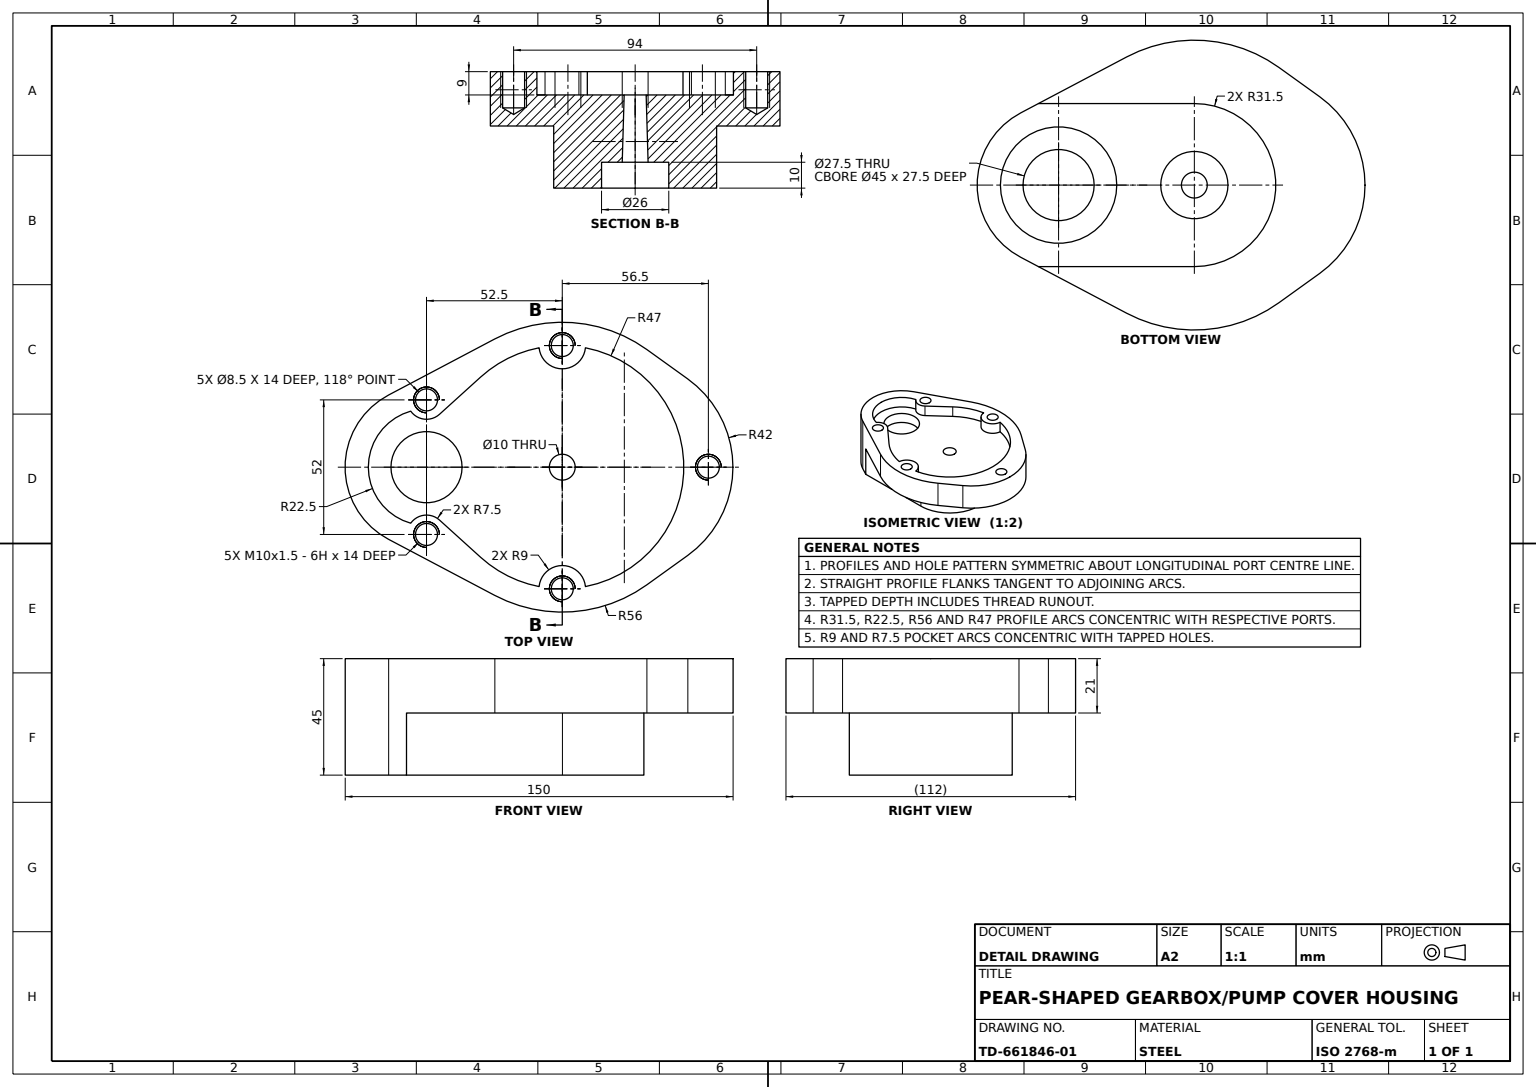
from build123d import *

# Parameters (mm, degrees)
FLANGE_BASE_21MM_DEPTH               = 21
PORT_POCKET_9MM_DEEP_DEPTH           = 9
TAPPED_HOLE_M10_DRILL_8_5_D          = 8.5
TAPPED_HOLE_M10_DRILL_8_5_DEPTH      = 14
TAPPED_HOLE_M10_DRILL_8_5_TIP        = 2.553657631
PORT_START                           = 24
PORT_BOSS_24MM_DEPTH                 = 24
SECONDARY_PORT_C_BORE_10_D           = 10
SECONDARY_PORT_C_BORE_10_DEPTH       = 99.679486355
SECONDARY_PORT_C_BORE_10_CBORE_D     = 26
SECONDARY_PORT_C_BORE_10_CBORE_DEPTH = 10


with BuildPart() as part:
    # Flange Base Profile → Flange Base 21mm (new body)
    with BuildSketch(Plane(origin=(0, 0, 0), x_dir=(1, 0, 0), z_dir=(0, 1, 0))):
        with BuildLine():
            Line((-49.528263536, 26.366666667), (-27.859648239, -14.7))
            ThreePointArc((-27.859648239, -14.7), (0, -31.5), (27.859648239, -14.7))
            Line((27.859648239, -14.7), (49.528263536, 26.366666667))
            ThreePointArc((49.528263536, 26.366666667), (55.868076531, 56.341617458), (45.485040276, 85.166666667))
            Line((45.485040276, 85.166666667), (34.113780207, 101))
            ThreePointArc((34.113780207, 101), (0, 118.5), (-34.113780207, 101))
            Line((-34.113780207, 101), (-45.485040276, 85.166666667))
            ThreePointArc((-45.485040276, 85.166666667), (-55.868076531, 56.341617458), (-49.528263536, 26.366666667))
        make_face()
    extrude(amount=FLANGE_BASE_21MM_DEPTH)

    # Port Pocket Profile → Port Pocket 9mm Deep (cut)
    with BuildSketch(Plane(origin=(0, 21, 0), x_dir=(1, 0, 0), z_dir=(0, 1, 0))):
        with BuildLine():
            Line((-21.596473004, 6.312079988), (-20.437807431, 5.031104632))
            ThreePointArc((-20.437807431, 5.031104632), (-18.544261668, -0.813612883), (-21.653846154, -6.112360162))
            ThreePointArc((-21.653846154, -6.112360162), (0, -22.5), (21.653846154, -6.112360162))
            ThreePointArc((21.653846154, -6.112360162), (18.544261668, -0.813612883), (20.437807431, 5.031104632))
            Line((20.437807431, 5.031104632), (34.856406768, 20.971744304))
            ThreePointArc((34.856406768, 20.971744304), (42.040245988, 31.485297592), (46.138297872, 43.541346672))
            ThreePointArc((46.138297872, 43.541346672), (38, 52.5), (46.138297872, 61.458653328))
            ThreePointArc((46.138297872, 61.458653328), (0, 99.5), (-46.138297872, 61.458653328))
            ThreePointArc((-46.138297872, 61.458653328), (-38, 52.5), (-46.138297872, 43.541346672))
            ThreePointArc((-46.138297872, 43.541346672), (-42.040245988, 31.485297592), (-34.856406768, 20.971744304))
            Line((-34.856406768, 20.971744304), (-21.596473004, 6.312079988))
        make_face()
    extrude(amount=-PORT_POCKET_9MM_DEEP_DEPTH, mode=Mode.SUBTRACT)

    # Tapped Hole M10 Drill Ø8.5
    with Locations(Plane(origin=(0, 21, -109), x_dir=(0, 0, 1), z_dir=(0, 1, 0))):
        with Locations((0, 0), (56.5, -47), (56.5, 47), (109, -26), (109, 26)):
            Hole(TAPPED_HOLE_M10_DRILL_8_5_D / 2, depth=TAPPED_HOLE_M10_DRILL_8_5_DEPTH)
            with Locations((0, 0, -(TAPPED_HOLE_M10_DRILL_8_5_DEPTH + TAPPED_HOLE_M10_DRILL_8_5_TIP / 2))):  # 118° drill point
                Cone(0, TAPPED_HOLE_M10_DRILL_8_5_D / 2, TAPPED_HOLE_M10_DRILL_8_5_TIP, mode=Mode.SUBTRACT)

    # Port Boss Profile → Port Boss 24mm (add)
    with BuildSketch(Plane.XZ.offset(PORT_START)):
        with BuildLine():
            Line((31.5, 0), (31.5, -52.5))
            ThreePointArc((31.5, -52.5), (0, -84), (-31.5, -52.5))
            Line((-31.5, -52.5), (-31.5, 0))
            Line((-31.5, 0), (-31.5, 7.800753774))
            Line((-31.5, 7.800753774), (-27.859648239, 14.7))
            ThreePointArc((-27.859648239, 14.7), (0, 31.5), (27.859648239, 14.7))
            Line((27.859648239, 14.7), (31.5, 7.800753774))
            Line((31.5, 7.800753774), (31.5, 0))
        make_face()
    extrude(amount=-PORT_BOSS_24MM_DEPTH)

    # Sketch7 → Main Port C-Bore Ø27.5 (revolve, cut)
    with BuildSketch(Plane(origin=(0, -24, 0), x_dir=(0, 0, -1), z_dir=(1, 0, 0))):
        Polygon((0, 0), (0, 99.616451954), (13.75, 99.616451954), (13.75, 27.5), (22.5, 27.5), (22.5, 0), align=None)
    revolve(axis=Axis((0, 86, 0), (0, -1, 0)), mode=Mode.SUBTRACT)

    # Secondary Port C-Bore Ø10
    with Locations(Plane(origin=(0, -24, -52.5), x_dir=(0, 0, -1), z_dir=(0, -1, 0))):
        with Locations((0, 0)):
            CounterBoreHole(SECONDARY_PORT_C_BORE_10_D / 2, SECONDARY_PORT_C_BORE_10_CBORE_D / 2, SECONDARY_PORT_C_BORE_10_CBORE_DEPTH, depth=SECONDARY_PORT_C_BORE_10_DEPTH)


solid = part.part
